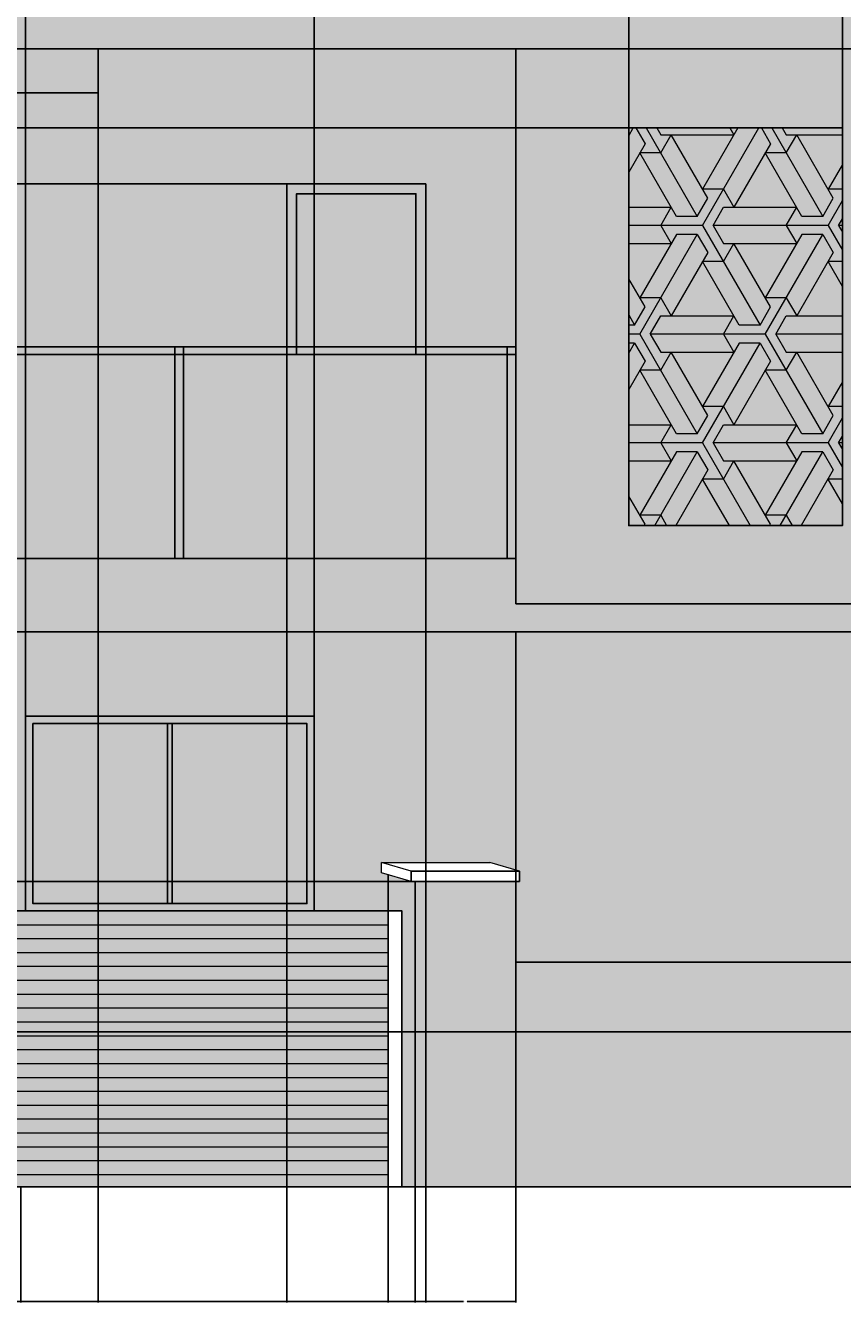
# Model space of a CAD drawing. Units: feet. Extents: x 2926 to 4178, y 965 to 1469.
# Tile 3 of 9: x 3068 to 3245, y 965 to 1241. Entities that reach past the tile are written whole.
import ezdxf

# ---------------------------------------------------------------- set-up
doc = ezdxf.new("R2010")
doc.units = ezdxf.units.FT
for name, color, linetype, lineweight in [('A-ANNO-DIMS', 2, 'Continuous', 18), ('A-ELEV', 7, 'Continuous', 25), ('A-ELEV-DETL', 8, 'Continuous', 18), ('A-ELEV-PATT', 9, 'Continuous', 13)]:
    doc.layers.add(name, color=color, linetype=linetype, lineweight=lineweight)
doc.styles.get("Standard").update_dxf_attribs({"font": 'arial.ttf'})
doc.dimstyles.get("Standard").update_dxf_attribs({"dimtxt": 0.18, "dimasz": 0.18, "dimexe": 0.18, "dimexo": 0.0625, "dimgap": 0.09, "dimtad": 0, "dimtih": 1, "dimtoh": 1, "dimdec": 1, "dimzin": 0, "dimdsep": 46, "dimlunit": 3, "dimtxsty": 'Standard', "dimcen": 0.09, "dimadec": 0, "dimazin": 0, "dimtfac": 1, "dimtdec": 1, "dimtofl": 0, "dimtmove": 0, "dimatfit": 3, "dimfxl": 1, "dimtolj": 1, "dimtzin": 0, "dimarcsym": 0})

# ---------------------------------------------------------------- blocks, each defined once
blk = doc.blocks.new('PILLAR-CAP-A')
for p, q in [((0, 2.25), (6.42, 4.14)), ((0, 2.25), (6.42, 4.14)), ((29.85, 4.14), (6.42, 4.14)), ((29.85, 4.14), (6.42, 4.14)), ((23.43, 2.25), (29.85, 4.14)), ((23.43, 2.25), (29.85, 4.14)), ((29.85, 1.89), (29.85, 4.14)), ((29.85, 1.89), (29.85, 4.14)), ((23.43, 0), (29.85, 1.89)), ((23.43, 0), (29.85, 1.89))]:
    blk.add_line(p, q)
blk = doc.blocks.new('*D12')
at = {"layer": 'A-ANNO-DIMS', "color": 0, "lineweight": -2, "transparency": 16777216}
for p, q in [((3335.85, 1023.86), (2926.57, 1023.86)), ((2926.75, 1023.68), (2926.75, 1007.27)), ((2926.75, 990.5), (2926.75, 1006.91)), ((2952.34, 990.32), (2926.57, 990.32))]:
    blk.add_line(p, q, dxfattribs=at)
at = {"layer": 'A-ANNO-DIMS', "color": 0, "transparency": 16777216}
for points in [[(2926.72, 1023.68), (2926.78, 1023.68), (2926.75, 1023.86)], [(2926.72, 990.5), (2926.78, 990.5), (2926.75, 990.32)]]:
    blk.add_solid(points, dxfattribs=at)
at = {"layer": 'Defpoints', "color": 0, "transparency": 16777216}
for p in [(2926.75, 1023.86), (3335.91, 1023.86), (2952.4, 990.32)]:
    blk.add_point(p, dxfattribs=at)
at = {"layer": 'A-ANNO-DIMS', "color": 0, "transparency": 16777216, "insert": (2926.75, 1007.09), "char_height": 0.18, "attachment_point": 5}
blk.add_mtext('\\A1;33.53', dxfattribs=at)
blk = doc.blocks.new('*D13')
at = {"layer": 'A-ANNO-DIMS', "color": 0, "lineweight": -2, "transparency": 16777216}
for p, q in [((3068.25, 1049.98), (2926.57, 1049.98)), ((2926.75, 1049.8), (2926.75, 1037.1)), ((2926.75, 1024.04), (2926.75, 1036.74)), ((3335.85, 1023.86), (2926.57, 1023.86))]:
    blk.add_line(p, q, dxfattribs=at)
at = {"layer": 'A-ANNO-DIMS', "color": 0, "transparency": 16777216}
for points in [[(2926.72, 1049.8), (2926.78, 1049.8), (2926.75, 1049.98)], [(2926.72, 1024.04), (2926.78, 1024.04), (2926.75, 1023.86)]]:
    blk.add_solid(points, dxfattribs=at)
at = {"layer": 'Defpoints', "color": 0, "transparency": 16777216}
for p in [(2926.75, 1049.98), (3068.31, 1049.98), (3335.91, 1023.86)]:
    blk.add_point(p, dxfattribs=at)
at = {"layer": 'A-ANNO-DIMS', "color": 0, "transparency": 16777216, "insert": (2926.75, 1036.92), "char_height": 0.18, "attachment_point": 5}
blk.add_mtext('\\A1;26.13', dxfattribs=at)
blk = doc.blocks.new('*D16')
at = {"layer": 'A-ANNO-DIMS', "color": 0, "lineweight": -2, "transparency": 16777216}
for p, q in [((3198.58, 1219.22), (2926.57, 1219.22)), ((2926.75, 1219.04), (2926.75, 1172.86)), ((2926.75, 1126.32), (2926.75, 1172.5)), ((2952.34, 1126.14), (2926.57, 1126.14))]:
    blk.add_line(p, q, dxfattribs=at)
at = {"layer": 'A-ANNO-DIMS', "color": 0, "transparency": 16777216}
for points in [[(2926.72, 1219.04), (2926.78, 1219.04), (2926.75, 1219.22)], [(2926.72, 1126.32), (2926.78, 1126.32), (2926.75, 1126.14)]]:
    blk.add_solid(points, dxfattribs=at)
at = {"layer": 'Defpoints', "color": 0, "transparency": 16777216}
for p in [(2926.75, 1219.22), (3198.64, 1219.22), (2952.4, 1126.14)]:
    blk.add_point(p, dxfattribs=at)
at = {"layer": 'A-ANNO-DIMS', "color": 0, "transparency": 16777216, "insert": (2926.75, 1172.68), "char_height": 0.18, "attachment_point": 5}
blk.add_mtext('\\A1;93.08', dxfattribs=at)
blk = doc.blocks.new('*D17')
at = {"layer": 'A-ANNO-DIMS', "color": 0, "lineweight": -2, "transparency": 16777216}
for p, q in [((2952.34, 1252.14), (2926.57, 1252.14)), ((2926.75, 1251.96), (2926.75, 1235.86)), ((2926.75, 1219.4), (2926.75, 1235.5)), ((3198.58, 1219.22), (2926.57, 1219.22))]:
    blk.add_line(p, q, dxfattribs=at)
at = {"layer": 'A-ANNO-DIMS', "color": 0, "transparency": 16777216}
for points in [[(2926.72, 1251.96), (2926.78, 1251.96), (2926.75, 1252.14)], [(2926.72, 1219.4), (2926.78, 1219.4), (2926.75, 1219.22)]]:
    blk.add_solid(points, dxfattribs=at)
at = {"layer": 'Defpoints', "color": 0, "transparency": 16777216}
for p in [(2926.75, 1252.14), (2952.4, 1252.14), (3198.64, 1219.22)]:
    blk.add_point(p, dxfattribs=at)
at = {"layer": 'A-ANNO-DIMS', "color": 0, "transparency": 16777216, "insert": (2926.75, 1235.68), "char_height": 0.18, "attachment_point": 5}
blk.add_mtext('\\A1;32.92', dxfattribs=at)
blk = doc.blocks.new('*D23')
at = {"layer": 'A-ANNO-DIMS', "color": 0, "lineweight": -2, "transparency": 16777216}
for p, q in [((3068.31, 1050.05), (3068.31, 1468.62)), ((3068.49, 1468.44), (3099.11, 1468.44)), ((3130.51, 1468.44), (3099.9, 1468.44)), ((3130.69, 1050.05), (3130.69, 1468.62))]:
    blk.add_line(p, q, dxfattribs=at)
at = {"layer": 'A-ANNO-DIMS', "color": 0, "transparency": 16777216}
for points in [[(3068.49, 1468.47), (3068.49, 1468.41), (3068.31, 1468.44)], [(3130.51, 1468.47), (3130.51, 1468.41), (3130.69, 1468.44)]]:
    blk.add_solid(points, dxfattribs=at)
at = {"layer": 'Defpoints', "color": 0, "transparency": 16777216}
for p in [(3130.69, 1468.44), (3068.31, 1049.98), (3130.69, 1049.98)]:
    blk.add_point(p, dxfattribs=at)
at = {"layer": 'A-ANNO-DIMS', "color": 0, "transparency": 16777216, "insert": (3099.5, 1468.44), "char_height": 0.18, "attachment_point": 5}
blk.add_mtext('\\A1;62.38', dxfattribs=at)
blk = doc.blocks.new('*D24')
at = {"layer": 'A-ANNO-DIMS', "color": 0, "lineweight": -2, "transparency": 16777216}
for p, q in [((3130.69, 1050.05), (3130.69, 1468.62)), ((3130.87, 1468.44), (3164.27, 1468.44)), ((3198.46, 1468.44), (3165.06, 1468.44)), ((3198.64, 1133.35), (3198.64, 1468.62))]:
    blk.add_line(p, q, dxfattribs=at)
at = {"layer": 'A-ANNO-DIMS', "color": 0, "transparency": 16777216}
for points in [[(3130.87, 1468.47), (3130.87, 1468.41), (3130.69, 1468.44)], [(3198.46, 1468.47), (3198.46, 1468.41), (3198.64, 1468.44)]]:
    blk.add_solid(points, dxfattribs=at)
at = {"layer": 'Defpoints', "color": 0, "transparency": 16777216}
for p in [(3198.64, 1468.44), (3198.64, 1133.29), (3130.69, 1049.98)]:
    blk.add_point(p, dxfattribs=at)
at = {"layer": 'A-ANNO-DIMS', "color": 0, "transparency": 16777216, "insert": (3164.67, 1468.44), "char_height": 0.18, "attachment_point": 5}
blk.add_mtext('\\A1;67.95', dxfattribs=at)
blk = doc.blocks.new('*D25')
at = {"layer": 'A-ANNO-DIMS', "color": 0, "lineweight": -2, "transparency": 16777216}
for p, q in [((3198.64, 1133.35), (3198.64, 1468.62)), ((3198.82, 1468.44), (3221.33, 1468.44)), ((3244.64, 1468.44), (3222.13, 1468.44)), ((3244.82, 1133.35), (3244.82, 1468.62))]:
    blk.add_line(p, q, dxfattribs=at)
at = {"layer": 'A-ANNO-DIMS', "color": 0, "transparency": 16777216}
for points in [[(3198.82, 1468.47), (3198.82, 1468.41), (3198.64, 1468.44)], [(3244.64, 1468.47), (3244.64, 1468.41), (3244.82, 1468.44)]]:
    blk.add_solid(points, dxfattribs=at)
at = {"layer": 'Defpoints', "color": 0, "transparency": 16777216}
for p in [(3244.82, 1468.44), (3198.64, 1133.29), (3244.82, 1133.29)]:
    blk.add_point(p, dxfattribs=at)
at = {"layer": 'A-ANNO-DIMS', "color": 0, "transparency": 16777216, "insert": (3221.73, 1468.44), "char_height": 0.18, "attachment_point": 5}
blk.add_mtext('\\A1;46.18', dxfattribs=at)
blk = doc.blocks.new('*D54')
at = {"layer": 'A-ANNO-DIMS', "color": 0, "lineweight": -2, "transparency": 16777216}
for p, q in [((3004.93, 1228.4), (3004.93, 965.34)), ((3084.03, 1170.16), (3084.03, 965.34)), ((3005.11, 965.52), (3044.17, 965.52)), ((3083.85, 965.52), (3044.79, 965.52))]:
    blk.add_line(p, q, dxfattribs=at)
at = {"layer": 'A-ANNO-DIMS', "color": 0, "transparency": 16777216}
for points in [[(3005.11, 965.55), (3005.11, 965.49), (3004.93, 965.52)], [(3083.85, 965.55), (3083.85, 965.49), (3084.03, 965.52)]]:
    blk.add_solid(points, dxfattribs=at)
at = {"layer": 'Defpoints', "color": 0, "transparency": 16777216}
for p in [(3004.93, 1228.46), (3084.03, 1170.22), (3084.03, 965.52)]:
    blk.add_point(p, dxfattribs=at)
at = {"layer": 'A-ANNO-DIMS', "color": 0, "transparency": 16777216, "insert": (3044.48, 965.52), "char_height": 0.18, "attachment_point": 5}
blk.add_mtext('\\A1;79.1', dxfattribs=at)
blk = doc.blocks.new('*D55')
at = {"layer": 'A-ANNO-DIMS', "color": 0, "lineweight": -2, "transparency": 16777216}
for p, q in [((3084.03, 1170.16), (3084.03, 965.34)), ((3124.76, 1170.16), (3124.76, 965.34)), ((3084.21, 965.52), (3104, 965.52)), ((3124.58, 965.52), (3104.79, 965.52))]:
    blk.add_line(p, q, dxfattribs=at)
at = {"layer": 'A-ANNO-DIMS', "color": 0, "transparency": 16777216}
for points in [[(3084.21, 965.55), (3084.21, 965.49), (3084.03, 965.52)], [(3124.58, 965.55), (3124.58, 965.49), (3124.76, 965.52)]]:
    blk.add_solid(points, dxfattribs=at)
at = {"layer": 'Defpoints', "color": 0, "transparency": 16777216}
for p in [(3084.03, 1170.22), (3124.76, 1170.22), (3124.76, 965.52)]:
    blk.add_point(p, dxfattribs=at)
at = {"layer": 'A-ANNO-DIMS', "color": 0, "transparency": 16777216, "insert": (3104.39, 965.52), "char_height": 0.18, "attachment_point": 5}
blk.add_mtext('\\A1;40.73', dxfattribs=at)
blk = doc.blocks.new('*D56')
at = {"layer": 'A-ANNO-DIMS', "color": 0, "lineweight": -2, "transparency": 16777216}
for p, q in [((3124.76, 1170.16), (3124.76, 965.34)), ((3154.77, 1170.16), (3154.77, 965.34)), ((3124.94, 965.52), (3139.3, 965.52)), ((3154.59, 965.52), (3140.23, 965.52))]:
    blk.add_line(p, q, dxfattribs=at)
at = {"layer": 'A-ANNO-DIMS', "color": 0, "transparency": 16777216}
for points in [[(3124.94, 965.55), (3124.94, 965.49), (3124.76, 965.52)], [(3154.59, 965.55), (3154.59, 965.49), (3154.77, 965.52)]]:
    blk.add_solid(points, dxfattribs=at)
at = {"layer": 'Defpoints', "color": 0, "transparency": 16777216}
for p in [(3124.76, 1170.22), (3154.77, 1170.22), (3154.77, 965.52)]:
    blk.add_point(p, dxfattribs=at)
at = {"layer": 'A-ANNO-DIMS', "color": 0, "transparency": 16777216, "insert": (3139.77, 965.52), "char_height": 0.18, "attachment_point": 5}
blk.add_mtext('\\A1;30.015', dxfattribs=at)
blk = doc.blocks.new('*D57')
at = {"layer": 'A-ANNO-DIMS', "color": 0, "lineweight": -2, "transparency": 16777216}
for p, q in [((3154.71, 1207.11), (2926.57, 1207.11)), ((2926.75, 1206.93), (2926.75, 1188.84)), ((2926.75, 1170.4), (2926.75, 1188.48)), ((3154.71, 1170.22), (2926.57, 1170.22))]:
    blk.add_line(p, q, dxfattribs=at)
at = {"layer": 'A-ANNO-DIMS', "color": 0, "transparency": 16777216}
for points in [[(2926.72, 1206.93), (2926.78, 1206.93), (2926.75, 1207.11)], [(2926.72, 1170.4), (2926.78, 1170.4), (2926.75, 1170.22)]]:
    blk.add_solid(points, dxfattribs=at)
at = {"layer": 'Defpoints', "color": 0, "transparency": 16777216}
for p in [(2926.75, 1207.11), (3154.77, 1207.11), (3154.77, 1170.22)]:
    blk.add_point(p, dxfattribs=at)
at = {"layer": 'A-ANNO-DIMS', "color": 0, "transparency": 16777216, "insert": (2926.75, 1188.66), "char_height": 0.18, "attachment_point": 5}
blk.add_mtext('\\A1;36.89', dxfattribs=at)
blk = doc.blocks.new('*D70')
at = {"layer": 'A-ANNO-DIMS', "color": 0, "lineweight": -2, "transparency": 16777216}
for p, q in [((3067.27, 990.26), (3067.27, 965.34)), ((3146.65, 990.26), (3146.65, 965.34)), ((3067.45, 965.52), (3106.57, 965.52)), ((3146.47, 965.52), (3107.35, 965.52))]:
    blk.add_line(p, q, dxfattribs=at)
at = {"layer": 'A-ANNO-DIMS', "color": 0, "transparency": 16777216}
for points in [[(3067.45, 965.55), (3067.45, 965.49), (3067.27, 965.52)], [(3146.47, 965.55), (3146.47, 965.49), (3146.65, 965.52)]]:
    blk.add_solid(points, dxfattribs=at)
at = {"layer": 'Defpoints', "color": 0, "transparency": 16777216}
for p in [(3067.27, 990.32), (3146.65, 990.32), (3146.65, 965.52)]:
    blk.add_point(p, dxfattribs=at)
at = {"layer": 'A-ANNO-DIMS', "color": 0, "transparency": 16777216, "insert": (3106.96, 965.52), "char_height": 0.18, "attachment_point": 5}
blk.add_mtext('\\A1;79.38', dxfattribs=at)
blk = doc.blocks.new('*D71')
at = {"layer": 'A-ANNO-DIMS', "color": 0, "lineweight": -2, "transparency": 16777216}
for p, q in [((3146.65, 990.26), (3146.65, 965.34)), ((3152.5, 990.26), (3152.5, 965.34)), ((3146.83, 965.52), (3149.18, 965.52)), ((3152.32, 965.52), (3149.97, 965.52))]:
    blk.add_line(p, q, dxfattribs=at)
at = {"layer": 'A-ANNO-DIMS', "color": 0, "transparency": 16777216}
for points in [[(3146.83, 965.55), (3146.83, 965.49), (3146.65, 965.52)], [(3152.32, 965.55), (3152.32, 965.49), (3152.5, 965.52)]]:
    blk.add_solid(points, dxfattribs=at)
at = {"layer": 'Defpoints', "color": 0, "transparency": 16777216}
for p in [(3146.65, 990.32), (3152.5, 990.32), (3152.5, 965.52)]:
    blk.add_point(p, dxfattribs=at)
at = {"layer": 'A-ANNO-DIMS', "color": 0, "transparency": 16777216, "insert": (3149.57, 965.52), "char_height": 0.18, "attachment_point": 5}
blk.add_mtext('\\A1;5.849', dxfattribs=at)
blk = doc.blocks.new('*D72')
at = {"layer": 'A-ANNO-DIMS', "color": 0, "lineweight": -2, "transparency": 16777216}
for p, q in [((3152.5, 990.26), (3152.5, 965.34)), ((3174.22, 990.26), (3174.22, 965.34)), ((3152.68, 965.52), (3162.96, 965.52)), ((3174.04, 965.52), (3163.75, 965.52))]:
    blk.add_line(p, q, dxfattribs=at)
at = {"layer": 'A-ANNO-DIMS', "color": 0, "transparency": 16777216}
for points in [[(3152.68, 965.55), (3152.68, 965.49), (3152.5, 965.52)], [(3174.04, 965.55), (3174.04, 965.49), (3174.22, 965.52)]]:
    blk.add_solid(points, dxfattribs=at)
at = {"layer": 'Defpoints', "color": 0, "transparency": 16777216}
for p in [(3152.5, 990.32), (3174.22, 990.32), (3174.22, 965.52)]:
    blk.add_point(p, dxfattribs=at)
at = {"layer": 'A-ANNO-DIMS', "color": 0, "transparency": 16777216, "insert": (3163.36, 965.52), "char_height": 0.18, "attachment_point": 5}
blk.add_mtext('\\A1;21.72', dxfattribs=at)
blk = doc.blocks.new('*D73')
at = {"layer": 'A-ANNO-DIMS', "color": 0, "lineweight": -2, "transparency": 16777216}
for p, q in [((3174.15, 1056.32), (2926.57, 1056.32)), ((2926.75, 1056.14), (2926.75, 1023.5)), ((2926.75, 990.5), (2926.75, 1023.14)), ((3174.15, 990.32), (2926.57, 990.32))]:
    blk.add_line(p, q, dxfattribs=at)
at = {"layer": 'A-ANNO-DIMS', "color": 0, "transparency": 16777216}
for points in [[(2926.72, 1056.14), (2926.78, 1056.14), (2926.75, 1056.32)], [(2926.72, 990.5), (2926.78, 990.5), (2926.75, 990.32)]]:
    blk.add_solid(points, dxfattribs=at)
at = {"layer": 'Defpoints', "color": 0, "transparency": 16777216}
for p in [(2926.75, 1056.32), (3174.22, 1056.32), (3174.22, 990.32)]:
    blk.add_point(p, dxfattribs=at)
at = {"layer": 'A-ANNO-DIMS', "color": 0, "transparency": 16777216, "insert": (2926.75, 1023.32), "char_height": 0.18, "attachment_point": 5}
blk.add_mtext('\\A1;66', dxfattribs=at)

msp = doc.modelspace()

# ---------------------------------------------------------------- hatches: boundary and pattern name
at = {"layer": 'A-ELEV-PATT'}
h = msp.add_hatch(color=256, dxfattribs=at)
h.dxf.hatch_style = 1
h.paths.add_polyline_path([(2968.9852, 1110.3246), (2958.1139, 1110.3246), (2958.1139, 1060.462), (2968.9852, 1060.462)])
h.paths.add_polyline_path([(3174.217, 1126.1389), (2952.4018, 1126.1389), (2952.4018, 1110.3246), (3174.217, 1110.3246), (3273.5987, 1110.3246), (3273.5987, 1116.3246), (3174.217, 1116.3246)], flags=17)
h.paths.add_polyline_path([(3289.413, 1252.1389), (2952.4018, 1252.1389), (2952.4018, 1236.3246), (3273.5987, 1236.3246), (3273.5987, 1110.3246), (3289.413, 1110.3246)])
h.paths.add_polyline_path([(3221.3497, 1355.2778), (3042.9199, 1355.2778), (3042.9199, 1339.4635), (3221.3497, 1339.4635)])
h.paths.add_polyline_path([(3379.9311, 1355.2778), (3262.1646, 1355.2778), (3262.1646, 1339.4635), (3364.1168, 1339.4635), (3364.1168, 990.3246), (3379.9311, 990.3246)])
h.paths.add_polyline_path([(3364.1168, 1330.7444), (3335.9143, 1330.7444), (3335.9143, 1023.8561), (3364.1168, 1023.8561), (3364.1168, 1027.6935), (3339.7517, 1027.6935), (3339.7517, 1326.907), (3364.1168, 1326.907)], flags=17)
h.paths.add_polyline_path([(3438.5707, 1443.6445), (3153.6951, 1443.6445), (3153.6951, 1427.8302), (3438.5707, 1427.8302)])
h.paths.add_polyline_path([(3174.217, 1427.8302), (3153.6951, 1427.8302), (3174.217, 1356.4366)])
h.paths.add_polyline_path([(3174.217, 1339.4635), (3042.9199, 1339.4635), (3070.6809, 1317.1829), (3174.217, 1317.1829)])
h.paths.add_polyline_path([(3244.819, 1219.2195), (3198.6415, 1219.2195), (3198.6415, 1133.2879), (3244.819, 1133.2879)], flags=17)
h = msp.add_hatch(color=256, dxfattribs=at)
h.dxf.hatch_style = 1
h.paths.add_polyline_path([(3006.649, 1296.2176), (2952.4018, 1296.2176), (2952.4018, 1252.1389), (3006.649, 1252.1389)])
h.paths.add_polyline_path([(3084.0314, 1226.8042), (3008.2802, 1226.8042), (3008.2802, 1171.8963), (3084.0314, 1171.8963)])
h.paths.add_polyline_path([(3004.9276, 1228.4641), (2995.6704, 1228.4641), (2995.6704, 1171.8963), (3004.9276, 1171.8963)])
h.paths.add_polyline_path([(3174.217, 1236.3246), (3084.0314, 1236.3246), (3084.0314, 1171.8963), (3124.7575, 1171.8963), (3124.7575, 1207.1083), (3154.7729, 1207.1083), (3154.7729, 1171.8963), (3174.217, 1171.8963)])
h.paths.add_polyline_path([(3273.5987, 1236.3246), (3174.217, 1236.3246), (3174.217, 1171.8963), (3174.217, 1126.1389), (3174.217, 1116.3246), (3273.5987, 1116.3246)], flags=16)
h.paths.add_polyline_path([(3198.6415, 1219.2195), (3244.819, 1219.2195), (3244.819, 1133.2879), (3198.6415, 1133.2879)], flags=0)
h.paths.add_polyline_path([(3432.4018, 1427.8302), (3174.217, 1427.8302), (3174.217, 1356.4366), (3174.5501, 1355.2778), (3221.3497, 1355.2778), (3221.3497, 1364.3965), (3232.8063, 1364.3965), (3232.8063, 1355.2778), (3236.4098, 1355.2778), (3236.4098, 1364.3965), (3247.8663, 1364.3965), (3247.8663, 1355.2778), (3250.7081, 1355.2778), (3250.7081, 1364.3965), (3262.1646, 1364.3965), (3262.1646, 1355.2778), (3379.9311, 1355.2778), (3379.9311, 990.3246), (3432.4018, 990.3246)])
h.paths.add_polyline_path([(3068.3128, 1092.0439), (3130.6886, 1092.0439), (3130.6886, 1049.9841), (3146.6469, 1049.9841), (3146.6469, 1057.7915), (3145.2184, 1058.2122), (3145.2184, 1060.462), (3168.644, 1060.462), (3174.217, 1058.8204), (3174.217, 1110.3246), (3004.9276, 1110.3246), (3004.9276, 1049.9841), (3068.3128, 1049.9841)])
h.paths.add_polyline_path([(3174.217, 1056.3197), (3152.4954, 1056.3197), (3152.4954, 990.3246), (3174.217, 990.3246)])
h.paths.add_polyline_path([(2974.1234, 1056.3197), (2952.4018, 1056.3197), (2952.4018, 990.3246), (2974.1234, 990.3246)])
h.paths.add_polyline_path([(3004.9276, 1110.3246), (2995.6704, 1110.3246), (2995.6704, 1049.9841), (3004.9276, 1049.9841)])
h = msp.add_hatch(color=256, dxfattribs=at)
h.dxf.hatch_style = 1
h.paths.add_polyline_path([(3335.9143, 1330.7444), (3364.1168, 1330.7444), (3364.1168, 1339.4635), (3262.1646, 1339.4635), (3262.1646, 1291.7348), (3250.7081, 1291.7348), (3250.7081, 1339.4635), (3247.8663, 1339.4635), (3247.8663, 1291.7348), (3236.4098, 1291.7348), (3236.4098, 1339.4635), (3232.8063, 1339.4635), (3232.8063, 1291.7348), (3221.3497, 1291.7348), (3221.3497, 1339.4635), (3174.217, 1339.4635), (3174.217, 1252.1389), (3289.413, 1252.1389), (3289.413, 1236.3246), (3289.413, 1110.3246), (3289.413, 1038.9216), (3174.217, 1038.9216), (3174.217, 990.3246), (3364.1168, 990.3246), (3364.1168, 1023.8561), (3335.9143, 1023.8561)])
h.paths.add_polyline_path([(3236.4098, 1355.2778), (3232.8063, 1355.2778), (3232.8063, 1339.4635), (3236.4098, 1339.4635)])
h.paths.add_polyline_path([(3250.7081, 1355.2778), (3247.8663, 1355.2778), (3247.8663, 1339.4635), (3250.7081, 1339.4635)])
h = msp.add_hatch(color=256, dxfattribs=at)
h.dxf.hatch_style = 1
h.paths.add_polyline_path([(3174.217, 1297.8963), (3172.3488, 1297.8963), (3006.649, 1297.8963), (3006.649, 1296.2176), (3087.9974, 1296.2176), (3087.9974, 1252.1389), (3089.8656, 1252.1389), (3089.8656, 1296.2176), (3172.3488, 1296.2176), (3172.3488, 1252.1389), (3174.217, 1252.1389)])
h.paths.add_polyline_path([(3102.4583, 1170.2176), (3172.3488, 1170.2176), (3172.3488, 1126.1389), (3174.217, 1126.1389), (3174.217, 1171.8963), (3172.3488, 1171.8963), (2952.4018, 1171.8963), (2952.4018, 1170.2176), (2952.4018, 1126.1389), (2954.27, 1126.1389), (2954.27, 1170.2176), (3100.5901, 1170.2176), (3100.5901, 1126.1389), (3102.4583, 1126.1389)])
h.paths.add_polyline_path([(3130.6886, 1092.0439), (3068.3128, 1092.0439), (3068.3128, 1049.9841), (3130.6886, 1049.9841)])
h.paths.add_polyline_path([(3099.0016, 1090.4638), (3099.0016, 1051.5643), (3069.893, 1051.5643), (3069.893, 1090.4638)], flags=16)
h.paths.add_polyline_path([(3099.9998, 1090.4638), (3129.1085, 1090.4638), (3129.1085, 1051.5643), (3099.9998, 1051.5643)], flags=16)
h.paths.add_polyline_path([(3067.2712, 1049.9841), (3060.102, 1049.9841), (3060.102, 990.3246), (3067.2712, 990.3246)])
h.paths.add_polyline_path([(3339.7517, 1326.907), (3364.1168, 1326.907), (3364.1168, 1330.7444), (3335.9143, 1330.7444), (3335.9143, 1023.8561), (3364.1168, 1023.8561), (3364.1168, 1027.6935), (3339.7517, 1027.6935)])
h.paths.add_polyline_path([(3154.7729, 1207.1083), (3124.7575, 1207.1083), (3124.7575, 1171.8963), (3126.8684, 1171.8963), (3126.8684, 1204.9974), (3152.6619, 1204.9974), (3152.6619, 1171.8963), (3154.7729, 1171.8963)])
h = msp.add_hatch(color=256, dxfattribs=at)
h.dxf.hatch_style = 1
h.paths.add_polyline_path([(3070.6809, 1296.2176), (3006.649, 1296.2176), (3006.649, 1252.1389), (3070.6809, 1252.1389)])
h.paths.add_polyline_path([(3087.9974, 1296.2176), (3070.6809, 1296.2176), (3070.6809, 1252.1389), (3087.9974, 1252.1389)])
h.paths.add_polyline_path([(3172.3488, 1296.2176), (3089.8656, 1296.2176), (3089.8656, 1252.1389), (3172.3488, 1252.1389)])
h.paths.add_polyline_path([(3152.6619, 1170.2176), (3126.8684, 1170.2176), (3126.8684, 1128.2498), (3152.6619, 1128.2498)], flags=17)
h.paths.add_polyline_path([(3152.6619, 1204.9974), (3126.8684, 1204.9974), (3126.8684, 1171.8963), (3152.6619, 1171.8963)])
h.paths.add_polyline_path([(3172.3488, 1170.2176), (3154.7729, 1170.2176), (3154.7729, 1126.1389), (3172.3488, 1126.1389)])
h.paths.add_polyline_path([(3154.7729, 1170.2176), (3152.6619, 1170.2176), (3152.6619, 1128.2498), (3126.8684, 1128.2498), (3126.8684, 1170.2176), (3124.7575, 1170.2176), (3124.7575, 1126.1389), (3154.7729, 1126.1389)])
h.paths.add_polyline_path([(3124.7575, 1170.2176), (3102.4583, 1170.2176), (3102.4583, 1126.1389), (3124.7575, 1126.1389)])
h.paths.add_polyline_path([(3100.5901, 1170.2176), (3084.0314, 1170.2176), (3084.0314, 1126.1389), (3100.5901, 1126.1389)])
h.paths.add_polyline_path([(3084.0314, 1170.2176), (3008.2802, 1170.2176), (3008.2802, 1126.1389), (3084.0314, 1126.1389)])
h.paths.add_polyline_path([(2995.6704, 1170.2176), (2971.1978, 1170.2176), (2971.1978, 1126.1389), (2995.6704, 1126.1389)])
h.paths.add_polyline_path([(3004.9276, 1170.2176), (2995.6704, 1170.2176), (2995.6704, 1126.1389), (3004.9276, 1126.1389)])
h.paths.add_polyline_path([(3364.1168, 1326.907), (3339.7517, 1326.907), (3339.7517, 1027.6935), (3364.1168, 1027.6935)])
h.paths.add_polyline_path([(3099.0016, 1090.4638), (3069.893, 1090.4638), (3069.893, 1051.5643), (3099.0016, 1051.5643)])
h.paths.add_polyline_path([(3129.1085, 1090.4638), (3099.9998, 1090.4638), (3099.9998, 1051.5643), (3129.1085, 1051.5643)])
h.paths.add_polyline_path([(2968.9852, 1170.2176), (2958.1139, 1170.2176), (2958.1139, 1126.1389), (2968.9852, 1126.1389)])
h.paths.add_polyline_path([(2958.1139, 1170.2176), (2954.27, 1170.2176), (2954.27, 1126.1389), (2958.1139, 1126.1389)])
h.paths.add_polyline_path([(2971.1978, 1170.2176), (2968.9852, 1170.2176), (2968.9852, 1126.1389), (2971.1978, 1126.1389)])
h = msp.add_hatch(color=256, dxfattribs=at)
h.dxf.hatch_style = 1
h.paths.add_polyline_path([(2971.1978, 1235.6728), (2968.9852, 1236.3246), (2968.9852, 1171.8963), (2971.1978, 1171.8963)])
h.paths.add_polyline_path([(2971.1978, 1109.6728), (2968.9852, 1110.3246), (2968.9852, 1060.462), (2971.1978, 1060.462)])
h.paths.add_polyline_path([(3084.0314, 1236.3246), (2968.9852, 1236.3246), (2995.6704, 1228.4641), (3004.9276, 1228.4641), (3008.2802, 1226.8042), (3084.0314, 1226.8042)])
h = msp.add_hatch(color=256, dxfattribs=at)
h.dxf.hatch_style = 1
h.paths.add_polyline_path([(2980.5295, 1057.9557), (2974.9754, 1056.3197), (2974.1234, 1056.3197), (2974.1234, 990.3246), (2977.7283, 990.3246), (2977.7283, 1049.9841), (2980.5295, 1049.9841)])
h.paths.add_polyline_path([(3152.4954, 1056.3197), (3151.6434, 1056.3197), (3146.6469, 1057.7915), (3146.6469, 1049.9841), (3149.6449, 1049.9841), (3149.6449, 990.3246), (3152.4954, 990.3246)])
h.paths.add_polyline_path([(3008.2802, 1226.8042), (3004.9276, 1228.4641), (3004.9276, 1171.8963), (3008.2802, 1171.8963)])
h = msp.add_hatch(dxfattribs=at)
h.set_pattern_fill('ESCHER', color=256, scale=0.89)
h.paths.add_polyline_path([(3244.819, 1219.2195), (3198.6415, 1219.2195), (3198.6415, 1133.2879), (3244.819, 1133.2879)])
h = msp.add_hatch(color=256, dxfattribs=at)
h.dxf.hatch_style = 1
h.paths.add_polyline_path([(3289.413, 1110.3246), (3174.217, 1110.3246), (3174.217, 1058.8204), (3175.069, 1058.5694), (3175.069, 1056.3197), (3174.217, 1056.3197), (3174.217, 1038.9216), (3289.413, 1038.9216)])
h = msp.add_hatch(color=256, dxfattribs=at)
h.dxf.hatch_style = 1
h.paths.add_polyline_path([(3146.6469, 1049.9841), (2980.5295, 1049.9841), (2980.5295, 990.3246), (3146.6469, 990.3246)])
h = msp.add_hatch(dxfattribs=at)
h.set_pattern_fill('_USER', color=256, scale=3, pattern_type=0)
h.set_pattern_definition([(0, (0, 0), (0, 3), [])])
h.paths.add_polyline_path([(3146.6469, 1049.9841), (2980.5295, 1049.9841), (2980.5295, 990.3246), (3146.6469, 990.3246)])

# ---------------------------------------------------------------- linework, layer by layer
at = {"layer": 'A-ELEV'}
for p, q in [((2952.4018, 1236.3246), (3273.5987, 1236.3246)), ((2952.4018, 1236.3246), (3273.5987, 1236.3246)), ((3174.217, 1116.3246), (3174.217, 1236.3246)), ((3174.217, 1116.3246), (3174.217, 1236.3246)), ((3008.2802, 1226.8042), (3084.0314, 1226.8042)), ((3008.2802, 1226.8042), (3084.0314, 1226.8042)), ((3174.217, 1116.3246), (3273.5987, 1116.3246)), ((3174.217, 1116.3246), (3273.5987, 1116.3246)), ((2952.4018, 1110.3246), (3289.413, 1110.3246)), ((2952.4018, 1110.3246), (3289.413, 1110.3246)), ((3174.217, 1110.3246), (3174.217, 990.3246)), ((3174.217, 1110.3246), (3174.217, 990.3246)), ((3146.6469, 1057.7915), (3146.6469, 990.3246)), ((3146.6469, 1057.7915), (3146.6469, 990.3246)), ((3289.413, 1038.9216), (3174.217, 1038.9216)), ((3289.413, 1038.9216), (3174.217, 1038.9216)), ((2952.4018, 990.3246), (3432.4018, 990.3246)), ((2952.4018, 990.3246), (3432.4018, 990.3246))]:
    msp.add_line(p, q, dxfattribs=at)
for points in [[(3289.413, 1236.3246), (3289.413, 1252.1389), (2952.4018, 1252.1389), (2952.4018, 1236.3246), (3273.5987, 1236.3246)], [(3289.413, 1236.3246), (3289.413, 1252.1389), (2952.4018, 1252.1389), (2952.4018, 1236.3246), (3273.5987, 1236.3246)], [(3084.0314, 1236.3246), (3174.217, 1236.3246), (3174.217, 1126.1389), (3084.0314, 1126.1389)], [(3084.0314, 1170.2176), (3084.0314, 1236.3246), (3174.217, 1236.3246), (3174.217, 1126.1389), (3084.0314, 1126.1389)], [(3124.7575, 1170.2176), (3124.7575, 1207.1083), (3154.7729, 1207.1083), (3154.7729, 1170.2176)], [(3126.8684, 1170.2176), (3126.8684, 1204.9974), (3152.6619, 1204.9974), (3152.6619, 1170.2176)], [(3174.217, 1110.3246), (2952.4018, 1110.3246), (2952.4018, 1126.1389), (3174.217, 1126.1389), (3174.217, 1116.3246)], [(3174.217, 1110.3246), (2952.4018, 1110.3246), (2952.4018, 1126.1389), (3174.217, 1126.1389), (3174.217, 1116.3246)], [(3154.7729, 1126.1389), (3124.7575, 1126.1389)]]:
    msp.add_lwpolyline(points, dxfattribs=at)
for points in [[(3198.6415, 1219.2195), (3244.819, 1219.2195), (3244.819, 1133.2879), (3198.6415, 1133.2879)], [(3198.6415, 1219.2195), (3244.819, 1219.2195), (3244.819, 1133.2879), (3198.6415, 1133.2879)], [(2952.4018, 1170.2176), (3174.217, 1170.2176), (3174.217, 1171.8963), (2952.4018, 1171.8963)], [(2952.4018, 1170.2176), (3174.217, 1170.2176), (3174.217, 1171.8963), (2952.4018, 1171.8963)], [(3100.5901, 1126.1389), (3102.4583, 1126.1389), (3102.4583, 1171.8963), (3100.5901, 1171.8963)], [(3100.5901, 1126.1389), (3102.4583, 1126.1389), (3102.4583, 1171.8963), (3100.5901, 1171.8963)], [(3172.3488, 1126.1389), (3174.217, 1126.1389), (3174.217, 1171.8963), (3172.3488, 1171.8963)], [(3172.3488, 1126.1389), (3174.217, 1126.1389), (3174.217, 1171.8963), (3172.3488, 1171.8963)], [(3068.3128, 1092.0439), (3130.6886, 1092.0439), (3130.6886, 1049.9841), (3068.3128, 1049.9841)], [(3068.3128, 1092.0439), (3130.6886, 1092.0439), (3130.6886, 1049.9841), (3068.3128, 1049.9841)], [(3069.893, 1090.4638), (3129.1085, 1090.4638), (3129.1085, 1051.5643), (3069.893, 1051.5643)], [(3069.893, 1090.4638), (3129.1085, 1090.4638), (3129.1085, 1051.5643), (3069.893, 1051.5643)], [(3099.0016, 1090.4638), (3099.9998, 1090.4638), (3099.9998, 1051.5643), (3099.0016, 1051.5643)], [(3099.0016, 1090.4638), (3099.9998, 1090.4638), (3099.9998, 1051.5643), (3099.0016, 1051.5643)], [(3175.069, 1056.3197), (3151.6434, 1056.3197), (3151.6434, 1058.5694), (3175.069, 1058.5694)], [(3175.069, 1056.3197), (3151.6434, 1056.3197), (3151.6434, 1058.5694), (3175.069, 1058.5694)], [(3174.217, 990.3246), (3152.4954, 990.3246), (3152.4954, 1056.3197), (3174.217, 1056.3197)], [(3174.217, 990.3246), (3152.4954, 990.3246), (3152.4954, 1056.3197), (3174.217, 1056.3197)], [(2977.7283, 1049.9841), (3149.6449, 1049.9841), (3149.6449, 990.3246), (2977.7283, 990.3246)], [(2977.7283, 1049.9841), (3149.6449, 1049.9841), (3149.6449, 990.3246), (2977.7283, 990.3246)]]:
    msp.add_lwpolyline(points, close=True, dxfattribs=at)

# ---------------------------------------------------------------- block references
at = {"layer": 'A-ELEV-DETL', "extrusion": (0, 0, -1), "zscale": -1}
msp.add_blockref('PILLAR-CAP-A', (-3175.0688, 1056.32), dxfattribs=at)

# ---------------------------------------------------------------- dimensions: what is measured, and where the dimension line sits
at = {"layer": 'A-ANNO-DIMS'}
for base, p1, p2, override, picture, middle in [((3130.6886, 1468.4445), (3068.3128, 1049.9841), (3130.6886, 1049.9841), {"dimdec": 2, "dimlfac": 1, "dimrnd": 0, "dimzin": 0, "dimdsep": 46, "dimlunit": 2}, '*D23', (3099.5007, 1468.4445)), ((3198.6415, 1468.4445), (3130.6886, 1049.9841), (3198.6415, 1133.2879), {"dimdec": 2, "dimlfac": 1, "dimrnd": 0, "dimzin": 0, "dimdsep": 46, "dimlunit": 2}, '*D24', (3164.6651, 1468.4445)), ((3244.819, 1468.4445), (3198.6415, 1133.2879), (3244.819, 1133.2879), {"dimdec": 2, "dimlfac": 1, "dimrnd": 0, "dimzin": 0, "dimdsep": 46, "dimlunit": 2}, '*D25', (3221.7303, 1468.4445)), ((3084.0314, 965.5246), (3004.9276, 1228.4641), (3084.0314, 1170.2176), {"dimdec": 1, "dimlfac": 1, "dimrnd": 0, "dimzin": 0, "dimdsep": 46, "dimlunit": 2}, '*D54', (3044.4795, 965.5246)), ((3124.7575, 965.5246), (3084.0314, 1170.2176), (3124.7575, 1170.2176), {"dimdec": 2, "dimlfac": 1, "dimrnd": 0, "dimzin": 0, "dimdsep": 46, "dimlunit": 2}, '*D55', (3104.3944, 965.5246)), ((3154.7729, 965.5246), (3124.7575, 1170.2176), (3154.7729, 1170.2176), {"dimdec": 3, "dimlfac": 1, "dimrnd": 0, "dimzin": 0, "dimdsep": 46, "dimlunit": 2}, '*D56', (3139.7652, 965.5246)), ((3146.6469, 965.5246), (3067.2712, 990.3246), (3146.6469, 990.3246), {"dimdec": 2, "dimlfac": 1, "dimrnd": 0, "dimzin": 0, "dimdsep": 46, "dimlunit": 2}, '*D70', (3106.959, 965.5246)), ((3152.49537, 965.524574), (3146.646866, 990.324574), (3152.49537, 990.324574), {"dimdec": 3, "dimlfac": 1, "dimrnd": 0, "dimzin": 0, "dimdsep": 46, "dimlunit": 2}, '*D71', (3149.571118, 965.524574)), ((3174.217, 965.5246), (3152.4954, 990.3246), (3174.217, 990.3246), {"dimdec": 2, "dimlfac": 1, "dimrnd": 0, "dimzin": 0, "dimdsep": 46, "dimlunit": 2}, '*D72', (3163.3562, 965.5246))]:
    dim = msp.add_linear_dim(base=base, p1=p1, p2=p2, dimstyle='Standard', override=override, dxfattribs=at)
    dim.commit()
    dim.dimension.update_dxf_attribs({"geometry": picture, "text_midpoint": middle})
for base, p1, p2, override, picture, middle in [((2926.7498, 1252.1389), (3198.6415, 1219.2195), (2952.4018, 1252.1389), {"dimdec": 2, "dimlfac": 1, "dimrnd": 0, "dimzin": 0, "dimdsep": 46, "dimlunit": 2}, '*D17', (2926.7498, 1235.6792)), ((2926.7498, 1219.2195), (2952.4018, 1126.1389), (3198.6415, 1219.2195), {"dimdec": 2, "dimlfac": 1, "dimrnd": 0, "dimzin": 0, "dimdsep": 46, "dimlunit": 2}, '*D16', (2926.7498, 1172.6792)), ((2926.7498, 1207.1083), (3154.7729, 1170.2176), (3154.7729, 1207.1083), {"dimdec": 2, "dimlfac": 1, "dimrnd": 0, "dimzin": 0, "dimdsep": 46, "dimlunit": 2}, '*D57', (2926.7498, 1188.663)), ((2926.7498, 1056.3197), (3174.217, 990.3246), (3174.217, 1056.3197), {"dimdec": 0, "dimlfac": 1, "dimrnd": 0, "dimzin": 0, "dimdsep": 46, "dimlunit": 2}, '*D73', (2926.7498, 1023.3221)), ((2926.7498, 1049.9841), (3335.9143, 1023.8561), (3068.3128, 1049.9841), {"dimdec": 2, "dimlfac": 1, "dimrnd": 0, "dimzin": 0, "dimdsep": 46, "dimlunit": 2}, '*D13', (2926.7498, 1036.9201)), ((2926.7498, 1023.8561), (2952.4018, 990.3246), (3335.9143, 1023.8561), {"dimdec": 2, "dimlfac": 1, "dimrnd": 0, "dimzin": 0, "dimdsep": 46, "dimlunit": 2}, '*D12', (2926.7498, 1007.0903))]:
    dim = msp.add_linear_dim(base=base, p1=p1, p2=p2, angle=90, dimstyle='Standard', override=override, dxfattribs=at)
    dim.commit()
    dim.dimension.update_dxf_attribs({"geometry": picture, "text_midpoint": middle})

doc.saveas('drawing.dxf')
